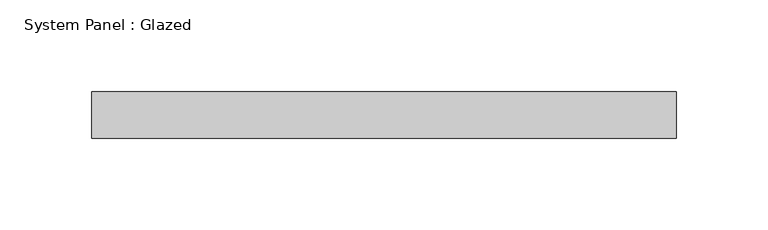
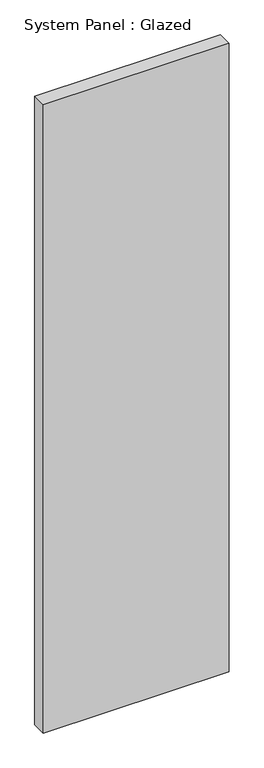
"""IFC4 building model written with IfcOpenShell, lengths in millimetres: plate geometry, System Panel : Glazed."""

from ifc_helpers import new_model, si_unit, origin, origin_with_axes, place, context, project, spatial, polyline, outline, extrude, source, transform, mapped, element, save


def system_panel_glazed_3c18516d(model_context):
    return source(origin(), model_context, "Body", "SweptSolid", [
        extrude(outline(polyline([(159.8083333, 19.05), (-159.8083333, 19.05), (-159.8083333, 44.45), (159.8083333, 44.45), (159.8083333, 19.05)])), origin_with_axes(), (0.0, 0.0, 1.0), 1143.0),
    ])


if __name__ == "__main__":
    model = new_model("IFC4")
    model_context = context("Model", 3, world=origin())
    ifc_project = project(units=[si_unit("LENGTHUNIT", "METRE", prefix="MILLI")], contexts=[model_context])
    site = spatial("IfcSite", under=ifc_project)
    building = spatial("IfcBuilding", under=site)
    placement = place(None, origin())
    system_panel_glazed_shape = system_panel_glazed_3c18516d(model_context)
    element("IfcPlate", 1, ObjectType="System Panel : Glazed", at=placement, inside=building, context=model_context, shape_type="MappedRepresentation", body=[
        mapped(system_panel_glazed_shape, transform((0.0, 0.0, 0.0), x_axis=(1.0, 0.0, 0.0), y_axis=(0.0, 1.0, 0.0), z_axis=(0.0, 0.0, 1.0))),
    ])
    save(model, "model.ifc")

# Revit data of these elements
# Type "System Panel : Glazed"
#   Construction Type Id = "GSP4R"
#   Analytic Construction = "1/8 in Pilkington single glazing"
#   Visual Light Transmittance = 0.9
#   Solar Heat Gain Coefficient = 0.86
#   Heat Transfer Coefficient (U) = 1.18115 BTU/(h·ft²·°F)
#   Define Thermal Properties by = 1
# Element 1 (IfcPlate, "System Panel : Glazed")
#   Materials on its faces: "Glass"
# Materials
#   "Glass": class "Glass", colour RGB 0 128 192, transparency 0.75, Description = "Soda Lime Glass", Cost = 0
